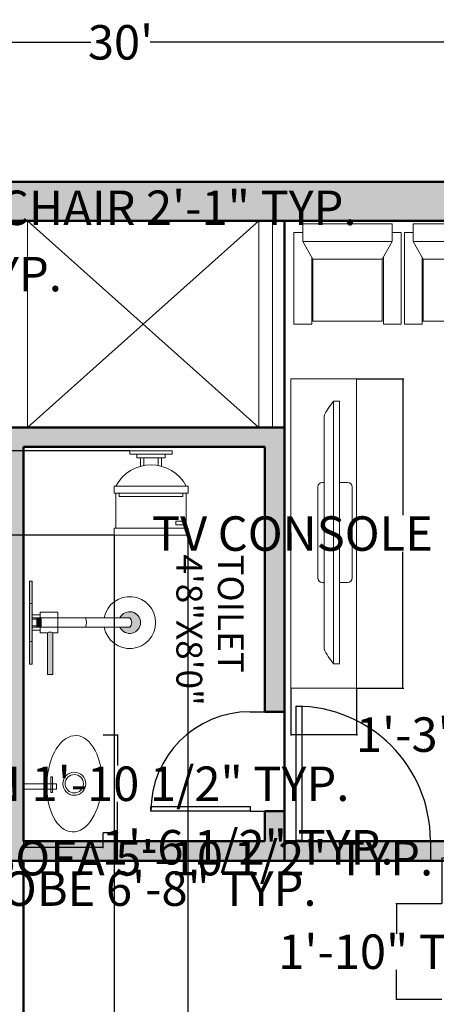
# Model space of a CAD drawing. Units: inches. Extents: x 22042254 to 25404563, y 17568978 to 17626777.
# Tile 43 of 45: x 22179940 to 22180037, y 17626547 to 17626775. Entities that reach past the tile are written whole.
import ezdxf

# ---------------------------------------------------------------- set-up
doc = ezdxf.new("R2010")
doc.units = ezdxf.units.IN
doc.header["$MEASUREMENT"] = 0
for name, color, linetype, lineweight in [('A-ANNO-DIMS', 2, 'Continuous', 18), ('A-AREA-IDEN', 7, 'Continuous', 18), ('A-FLOR-OPEN', 252, 'Continuous', 18), ('A-WALL-PATT', 244, 'Continuous', 13), ('doors', 4, 'Continuous', 25), ('furniture', 8, 'Continuous', 18), ('PLUMBING FIXTURES', 9, 'Continuous', 18), ('walls', 252, 'Continuous', 50)]:
    doc.layers.add(name, color=color, linetype=linetype, lineweight=lineweight)
doc.styles.get("Standard").update_dxf_attribs({"font": 'arial.ttf'})
doc.dimstyles.get("Standard").update_dxf_attribs({"dimtxt": 8, "dimasz": 0.18, "dimexe": 0.18, "dimexo": 0.0625, "dimgap": 0.09, "dimtad": 0, "dimtih": 1, "dimtoh": 1, "dimzin": 0, "dimdsep": 46, "dimlunit": 3, "dimtxsty": 'Standard', "dimcen": 0.09, "dimadec": 0, "dimazin": 0, "dimtfac": 1, "dimtofl": 0, "dimtmove": 0, "dimatfit": 3, "dimfxl": 1, "dimtolj": 1, "dimtzin": 0, "dimarcsym": 0})

# ---------------------------------------------------------------- blocks, each defined once
blk = doc.blocks.new('*D1')
at = {"layer": 'A-ANNO-DIMS', "color": 0, "lineweight": -2, "transparency": 16777216}
for p, q in [((22179783.73, 17626737.84), (22179783.73, 17626770.35)), ((22179783.91, 17626770.17), (22179956.86, 17626770.17)), ((22180143.55, 17626770.17), (22179970.61, 17626770.17)), ((22180143.73, 17626737.84), (22180143.73, 17626770.35))]:
    blk.add_line(p, q, dxfattribs=at)
at = {"layer": 'A-ANNO-DIMS', "color": 0, "transparency": 16777216}
for points in [[(22179783.91, 17626770.2), (22179783.91, 17626770.14), (22179783.73, 17626770.17)], [(22180143.55, 17626770.2), (22180143.55, 17626770.14), (22180143.73, 17626770.17)]]:
    blk.add_solid(points, dxfattribs=at)
at = {"layer": 'Defpoints', "color": 0, "transparency": 16777216}
for p in [(22180143.73, 17626770.17), (22179783.73, 17626737.78), (22180143.73, 17626737.78)]:
    blk.add_point(p, dxfattribs=at)
at = {"layer": 'A-ANNO-DIMS', "color": 0, "transparency": 16777216, "insert": (22179963.73, 17626770.17), "char_height": 8, "attachment_point": 5}
blk.add_mtext("\\A1;30'", dxfattribs=at)
blk = doc.blocks.new('FABRIC SOFA 1S')
at = {"layer": 'furniture'}
for p, q in [((3, 18.12), (34, 18.12)), ((3, 15.12), (3, 18.12)), ((34, 12.12), (34, 18.12)), ((0, -15.12), (0, 15.12)), ((6, 15.12), (0, 15.12)), ((6, -15.12), (6, 15.12)), ((12, 11.75), (6, 15.12)), ((11.33, 12.12), (34, 12.12)), ((6, -15.12), (12, -11.75)), ((11.33, -12.12), (34, -12.12)), ((34, -12.12), (34, -18.12)), ((6, -15.12), (0, -15.12)), ((3, -18.12), (3, -15.12)), ((3, -18.12), (34, -18.12))]:
    blk.add_line(p, q, dxfattribs=at)
blk.add_lwpolyline([(12, -11.75), (12, 11.75), (33, 11.75), (33, -11.75)], close=True, dxfattribs=at)
blk = doc.blocks.new('O.H SHOWER-PL')
at = {"layer": 'PLUMBING FIXTURES'}
for points in [[(-1.838, 0), (-1.838, -0.25), (1.838, -0.25), (1.838, 0)], [(0.461, -8.724), (0.461, -9.667, -0.422337), (-0.461, -9.667), (-0.461, -8.724, 4.325472)]]:
    blk.add_hatch(color=256, dxfattribs=at).paths.add_polyline_path(points)
for p, q in [((-1.838, 0), (-1.838, -0.25)), ((1.838, 0), (-1.838, 0)), ((1.838, 0), (1.838, -0.25)), ((1.838, -0.25), (-1.838, -0.25)), ((-0.461, -0.25), (-0.461, -9.667)), ((0.461, -0.25), (0.461, -9.667))]:
    blk.add_line(p, q, dxfattribs=at)
for centre, radius, start, end in [((0, -4.479), 1.033, 243.52996, 296.47004), ((0, -9.667), 2.501, 100.61004, 79.38997), ((0, -9.667), 1.049, 116.03487, 63.96515), ((0, -9.219), 0.643, 224.20776, 315.79224)]:
    blk.add_arc(centre, radius, start, end, dxfattribs=at)
blk = doc.blocks.new('DIVERTER-PL')
at = {"layer": 'PLUMBING FIXTURES'}
for points in [[(4, 0), (-4, 0), (-4, -0.25), (4, -0.25)], [(0.375, -1.144), (0.375, -0.704), (-0.375, -0.704), (-0.375, -1.144)], [(1, -1.751, 0.30818), (1, -2.251), (5, -2.251), (5, -1.751)]]:
    blk.add_hatch(color=256, dxfattribs=at).paths.add_polyline_path(points)
for p, q in [((-4, 0), (-4, -0.25)), ((-4, 0), (4, 0)), ((4, 0), (4, -0.25)), ((-4, -0.25), (4, -0.25)), ((-4, -0.25), (4, -0.25)), ((-0.75, -0.25), (-0.75, -1.05)), ((-0.375, -0.704), (0.375, -0.704)), ((-0.375, -0.704), (-0.375, -1.144)), ((-0.318, -0.704), (-0.318, -0.25)), ((0.318, -0.704), (0.318, -0.25)), ((0.375, -0.704), (0.375, -1.144)), ((0.75, -0.25), (0.75, -1.05)), ((-1, -1.05), (-0.375, -1.05)), ((-1, -1.05), (-1, -2.75)), ((-0.375, -1.144), (0.375, -1.144)), ((0.375, -1.05), (1, -1.05)), ((1, -1.05), (1, -1.751)), ((-1, -2.75), (1, -2.75)), ((1, -2.251), (1, -2.75))]:
    blk.add_line(p, q, dxfattribs=at)
at = {"layer": 'PLUMBING FIXTURES', "ltscale": 12}
for p, q in [((1, -1.751), (5, -1.751)), ((5, -2.251), (5, -1.751)), ((1, -2.251), (5, -2.251))]:
    blk.add_line(p, q, dxfattribs=at)
at = {"layer": 'PLUMBING FIXTURES'}
blk.add_arc((1.367, -2.001), 0.444, 145.74346, 214.25654, dxfattribs=at)
blk = doc.blocks.new('A$C7F153053')
at = {"layer": 'PLUMBING FIXTURES', "xscale": -1, "rotation": 270}
for name in ['DIVERTER-PL', 'O.H SHOWER-PL']:
    blk.add_blockref(name, (12.166, 4), dxfattribs=at)
blk = doc.blocks.new('Toilet - Imperial')
for p, q in [((-10, 22), (-10, 12)), ((-10, 21), (-7, 21)), ((-7, 20), (-10, 20)), ((-7, 21), (-7, 20)), ((10, 12), (10, 22)), ((10.5, 12), (-10.5, 12)), ((-10.5, 10), (-10.5, 12)), ((9, 13), (-9, 13)), ((-9, 13), (-9, 12)), ((9, 12), (9, 13)), ((10.5, 12), (10.5, 10)), ((10.5, 10), (-10.5, 10)), ((-3, 4.4065), (-3, 2)), ((-2, 2), (-2, 4.1658)), ((2, 4.1658), (2, 2)), ((3, 2), (3, 4.4065)), ((4, 2), (-4, 2)), ((-4, 2), (-4, 1)), ((4, 1), (4, 2))]:
    blk.add_line(p, q)
for points in [[(10.5, 22), (10.5, 24), (-10.5, 24), (-10.5, 22)], [(6, 0), (6, 1), (-6, 1), (-6, 0)]]:
    blk.add_lwpolyline(points, close=True)
blk.add_arc((0, 15.3333), 11.3333, 208.0725, 331.9275)
blk = doc.blocks.new('*U24')
for p, q in [((0, 0), (0, -6)), ((40, 0), (40, -6))]:
    blk.add_line(p, q)
blk.add_lwpolyline([(0, 0), (0, 40), (1.75, 40), (1.75, 0)], close=True)
blk.add_arc((0, 0), 40, 0, 90)
blk = doc.blocks.new('BASIN-OVAL-WITH-TAP')
for p, q in [((-11.77, 0), (-4.13, 0)), ((-5.47, 1.62), (-5.47, -2.04)), ((-5.06, 1.61), (-5.47, 1.61)), ((-5.06, -2.04), (-5.06, 1.61)), ((-4.13, 0), (-4.13, -1.24)), ((-4.13, -1.24), (-11.77, -1.24)), ((-5.47, -2.04), (-5.06, -2.04))]:
    blk.add_line(p, q)
for radius in [2.67, 2.13, 2.13, 2.13]:
    blk.add_circle((0, 0), radius)
blk.add_ellipse((0, 0), major_axis=(-0.46, -11.19), ratio=0.56899)
blk = doc.blocks.new('PLASMA-LARGE')
at = {"layer": 'furniture'}
for p, q in [((-7.26, 0), (7.26, 0)), ((-18.61, -1), (18.61, -1)), ((-8, -1), (-8, -0.74)), ((8, -1), (8, -0.74)), ((-21, -2.5), (21, -2.5)), ((-21, -2.5), (-21, -3.5)), ((21, -2.5), (21, -3.5)), ((-21, -3.5), (21, -3.5)), ((-8, -3.5), (-8, -4.76)), ((8, -3.5), (8, -4.76)), ((-7.26, -5.5), (7.26, -5.5))]:
    blk.add_line(p, q, dxfattribs=at)
for centre, radius, start, end in [((-7.26, -0.74), 0.744, 90, 180), ((7.26, -0.74), 0.744, 0, 90), ((-13.97, -11.05), 11.07, 114.7602, 129.4175), ((13.97, -11.05), 11.07, 50.5825, 65.2398), ((-7.26, -4.76), 0.744, 180, 270), ((7.26, -4.76), 0.744, 270, 0)]:
    blk.add_arc(centre, radius, start, end, dxfattribs=at)
blk = doc.blocks.new('TV-CONSOLE')
for p, q in [((8.99, 35.63), (-6.22, 35.63)), ((-6.22, 35.63), (-6.22, -36.14)), ((8.99, -36.14), (8.99, 35.63)), ((-6.22, -36.14), (8.99, -36.14))]:
    blk.add_line(p, q)
at = {"xscale": 1.450199298177205, "yscale": 1.450199298177205, "zscale": 1.450199298177205, "rotation": 90}
blk.add_blockref('PLASMA-LARGE', (0, 0), dxfattribs=at)
blk = doc.blocks.new('*D36')
at = {"layer": 'A-ANNO-DIMS', "color": 0, "lineweight": -2, "transparency": 16777216}
for p, q in [((22179884.69, 17626728.11), (22179884.69, 17626731.96)), ((22179884.87, 17626731.78), (22179909.36, 17626731.78)), ((22179909.54, 17626728.11), (22179909.54, 17626731.96)), ((22179909.54, 17626731.78), (22179909.72, 17626731.78))]:
    blk.add_line(p, q, dxfattribs=at)
at = {"layer": 'A-ANNO-DIMS', "color": 0, "transparency": 16777216}
for points in [[(22179884.87, 17626731.81), (22179884.87, 17626731.75), (22179884.69, 17626731.78)], [(22179909.36, 17626731.81), (22179909.36, 17626731.75), (22179909.54, 17626731.78)]]:
    blk.add_solid(points, dxfattribs=at)
at = {"layer": 'Defpoints', "color": 0, "transparency": 16777216}
for p in [(22179909.54, 17626731.78), (22179884.69, 17626728.05), (22179909.54, 17626728.05)]:
    blk.add_point(p, dxfattribs=at)
at = {"layer": 'A-ANNO-DIMS', "color": 0, "transparency": 16777216, "insert": (22179965.78, 17626731.78), "char_height": 8, "attachment_point": 5}
blk.add_mtext('\\A1;ARMCHAIR 2\'-1" TYP.', dxfattribs=at)
blk = doc.blocks.new('*D37')
at = {"layer": 'A-ANNO-DIMS', "color": 0, "lineweight": -2, "transparency": 16777216}
for p, q in [((22179909.6, 17626728.05), (22179913.44, 17626728.05)), ((22179913.26, 17626727.87), (22179913.26, 17626720.62)), ((22179913.26, 17626704.92), (22179913.26, 17626712.17)), ((22179909.6, 17626704.74), (22179913.44, 17626704.74))]:
    blk.add_line(p, q, dxfattribs=at)
at = {"layer": 'A-ANNO-DIMS', "color": 0, "transparency": 16777216}
for points in [[(22179913.23, 17626727.87), (22179913.29, 17626727.87), (22179913.26, 17626728.05)], [(22179913.23, 17626704.92), (22179913.29, 17626704.92), (22179913.26, 17626704.74)]]:
    blk.add_solid(points, dxfattribs=at)
at = {"layer": 'Defpoints', "color": 0, "transparency": 16777216}
for p in [(22179909.54, 17626728.05), (22179909.54, 17626704.74), (22179913.26, 17626704.74)]:
    blk.add_point(p, dxfattribs=at)
at = {"layer": 'A-ANNO-DIMS', "color": 0, "transparency": 16777216, "insert": (22179913.26, 17626716.39), "char_height": 8, "attachment_point": 5}
blk.add_mtext('\\A1;1\'-11 1/2" TYP.', dxfattribs=at)
blk = doc.blocks.new('*D38')
at = {"layer": 'A-ANNO-DIMS', "color": 0, "lineweight": -2, "transparency": 16777216}
for p, q in [((22180018.54, 17626692.07), (22180029.42, 17626692.07)), ((22180029.24, 17626691.89), (22180029.24, 17626660.42)), ((22180029.24, 17626620.49), (22180029.24, 17626651.96)), ((22180018.54, 17626620.31), (22180029.42, 17626620.31))]:
    blk.add_line(p, q, dxfattribs=at)
at = {"layer": 'A-ANNO-DIMS', "color": 0, "transparency": 16777216}
for points in [[(22180029.21, 17626691.89), (22180029.27, 17626691.89), (22180029.24, 17626692.07)], [(22180029.21, 17626620.49), (22180029.27, 17626620.49), (22180029.24, 17626620.31)]]:
    blk.add_solid(points, dxfattribs=at)
at = {"layer": 'Defpoints', "color": 0, "transparency": 16777216}
for p in [(22180018.48, 17626692.07), (22180029.24, 17626692.07), (22180018.48, 17626620.31)]:
    blk.add_point(p, dxfattribs=at)
at = {"layer": 'A-ANNO-DIMS', "color": 0, "transparency": 16777216, "insert": (22180029.24, 17626656.19), "char_height": 8, "attachment_point": 5}
blk.add_mtext('\\A1;TV CONSOLE 6\'-0" TYP.', dxfattribs=at)
blk = doc.blocks.new('*D39')
at = {"layer": 'A-ANNO-DIMS', "color": 0, "lineweight": -2, "transparency": 16777216}
for p, q in [((22180003.26, 17626620.25), (22180003.26, 17626609.36)), ((22180018.48, 17626620.25), (22180018.48, 17626609.36)), ((22180003.44, 17626609.54), (22180018.3, 17626609.54)), ((22180018.48, 17626609.54), (22180018.66, 17626609.54))]:
    blk.add_line(p, q, dxfattribs=at)
at = {"layer": 'A-ANNO-DIMS', "color": 0, "transparency": 16777216}
for points in [[(22180003.44, 17626609.57), (22180003.44, 17626609.51), (22180003.26, 17626609.54)], [(22180018.3, 17626609.57), (22180018.3, 17626609.51), (22180018.48, 17626609.54)]]:
    blk.add_solid(points, dxfattribs=at)
at = {"layer": 'Defpoints', "color": 0, "transparency": 16777216}
for p in [(22180003.26, 17626620.31), (22180018.48, 17626620.31), (22180018.48, 17626609.54)]:
    blk.add_point(p, dxfattribs=at)
at = {"layer": 'A-ANNO-DIMS', "color": 0, "transparency": 16777216, "insert": (22180042.75, 17626609.54), "char_height": 8, "attachment_point": 5}
blk.add_mtext('\\A1;1\'-3" TYP.', dxfattribs=at)
blk = doc.blocks.new('*D42')
at = {"layer": 'A-ANNO-DIMS', "color": 0, "lineweight": -2, "transparency": 16777216}
for p, q in [((22179814.6, 17626585.75), (22179814.6, 17626573.62)), ((22179894.63, 17626585.75), (22179894.63, 17626573.62)), ((22179814.78, 17626573.8), (22179894.45, 17626573.8)), ((22179894.63, 17626573.8), (22179894.81, 17626573.8))]:
    blk.add_line(p, q, dxfattribs=at)
at = {"layer": 'A-ANNO-DIMS', "color": 0, "transparency": 16777216}
for points in [[(22179814.78, 17626573.83), (22179814.78, 17626573.77), (22179814.6, 17626573.8)], [(22179894.45, 17626573.83), (22179894.45, 17626573.77), (22179894.63, 17626573.8)]]:
    blk.add_solid(points, dxfattribs=at)
at = {"layer": 'Defpoints', "color": 0, "transparency": 16777216}
for p in [(22179814.6, 17626585.81), (22179894.63, 17626585.81), (22179894.63, 17626573.8)]:
    blk.add_point(p, dxfattribs=at)
at = {"layer": 'A-ANNO-DIMS', "color": 0, "transparency": 16777216, "insert": (22179953.9, 17626573.8), "char_height": 8, "attachment_point": 5}
blk.add_mtext('\\A1;WARDROBE 6\'-8" TYP.', dxfattribs=at)
blk = doc.blocks.new('*D46')
at = {"layer": 'A-ANNO-DIMS', "color": 0, "lineweight": -2, "transparency": 16777216}
for p, q in [((22179959.69, 17626609.47), (22179963.21, 17626609.47)), ((22179963.03, 17626609.29), (22179963.03, 17626602.36)), ((22179963.03, 17626586.98), (22179963.03, 17626593.91)), ((22179959.69, 17626586.8), (22179963.21, 17626586.8))]:
    blk.add_line(p, q, dxfattribs=at)
at = {"layer": 'A-ANNO-DIMS', "color": 0, "transparency": 16777216}
for points in [[(22179963, 17626609.29), (22179963.06, 17626609.29), (22179963.03, 17626609.47)], [(22179963, 17626586.98), (22179963.06, 17626586.98), (22179963.03, 17626586.8)]]:
    blk.add_solid(points, dxfattribs=at)
at = {"layer": 'Defpoints', "color": 0, "transparency": 16777216}
for p in [(22179959.63, 17626609.47), (22179963.03, 17626609.47), (22179959.63, 17626586.8)]:
    blk.add_point(p, dxfattribs=at)
at = {"layer": 'A-ANNO-DIMS', "color": 0, "transparency": 16777216, "insert": (22179963.03, 17626598.14), "char_height": 8, "attachment_point": 5}
blk.add_mtext('\\A1;BASIN 1\'-10 1/2" TYP.', dxfattribs=at)
blk = doc.blocks.new('*D47')
at = {"layer": 'A-ANNO-DIMS', "color": 0, "lineweight": -2, "transparency": 16777216}
for p, q in [((22179941.23, 17626586.74), (22179941.23, 17626583.22)), ((22179959.63, 17626586.74), (22179959.63, 17626583.22)), ((22179941.41, 17626583.4), (22179959.45, 17626583.4)), ((22179959.63, 17626583.4), (22179959.81, 17626583.4))]:
    blk.add_line(p, q, dxfattribs=at)
at = {"layer": 'A-ANNO-DIMS', "color": 0, "transparency": 16777216}
for points in [[(22179941.41, 17626583.43), (22179941.41, 17626583.37), (22179941.23, 17626583.4)], [(22179959.45, 17626583.43), (22179959.45, 17626583.37), (22179959.63, 17626583.4)]]:
    blk.add_solid(points, dxfattribs=at)
at = {"layer": 'Defpoints', "color": 0, "transparency": 16777216}
for p in [(22179941.23, 17626586.8), (22179959.63, 17626586.8), (22179959.63, 17626583.4)]:
    blk.add_point(p, dxfattribs=at)
at = {"layer": 'A-ANNO-DIMS', "color": 0, "transparency": 16777216, "insert": (22179993.22, 17626583.4), "char_height": 8, "attachment_point": 5}
blk.add_mtext('\\A1;1\'-6 1/2" TYP.', dxfattribs=at)
blk = doc.blocks.new('*D48')
at = {"layer": 'A-ANNO-DIMS', "color": 0, "lineweight": -2, "transparency": 16777216}
for p, q in [((22180038.35, 17626580.87), (22180038.17, 17626580.87)), ((22180038.35, 17626570.34), (22180038.35, 17626581.05)), ((22180108.78, 17626580.87), (22180038.53, 17626580.87)), ((22180108.96, 17626570.34), (22180108.96, 17626581.05))]:
    blk.add_line(p, q, dxfattribs=at)
at = {"layer": 'A-ANNO-DIMS', "color": 0, "transparency": 16777216}
for points in [[(22180038.53, 17626580.9), (22180038.53, 17626580.84), (22180038.35, 17626580.87)], [(22180108.78, 17626580.9), (22180108.78, 17626580.84), (22180108.96, 17626580.87)]]:
    blk.add_solid(points, dxfattribs=at)
at = {"layer": 'Defpoints', "color": 0, "transparency": 16777216}
for p in [(22180038.35, 17626580.87), (22180038.35, 17626570.27), (22180108.96, 17626570.27)]:
    blk.add_point(p, dxfattribs=at)
at = {"layer": 'A-ANNO-DIMS', "color": 0, "transparency": 16777216, "insert": (22179984.52, 17626580.87), "char_height": 8, "attachment_point": 5}
blk.add_mtext('\\A1;SOFA 5\'-10 1/2" TYP.', dxfattribs=at)
blk = doc.blocks.new('*D49')
at = {"layer": 'A-ANNO-DIMS', "color": 0, "lineweight": -2, "transparency": 16777216}
for p, q in [((22180038.29, 17626570.27), (22180027.58, 17626570.27)), ((22180027.76, 17626570.09), (22180027.76, 17626563.33)), ((22180027.76, 17626548.22), (22180027.76, 17626554.98)), ((22180038.29, 17626548.04), (22180027.58, 17626548.04))]:
    blk.add_line(p, q, dxfattribs=at)
at = {"layer": 'A-ANNO-DIMS', "color": 0, "transparency": 16777216}
for points in [[(22180027.73, 17626570.09), (22180027.79, 17626570.09), (22180027.76, 17626570.27)], [(22180027.73, 17626548.22), (22180027.79, 17626548.22), (22180027.76, 17626548.04)]]:
    blk.add_solid(points, dxfattribs=at)
at = {"layer": 'Defpoints', "color": 0, "transparency": 16777216}
for p in [(22180038.35, 17626570.27), (22180027.76, 17626548.04), (22180038.35, 17626548.04)]:
    blk.add_point(p, dxfattribs=at)
at = {"layer": 'A-ANNO-DIMS', "color": 0, "transparency": 16777216, "insert": (22180027.76, 17626559.16), "char_height": 8, "attachment_point": 5}
blk.add_mtext('\\A1;1\'-10" TYP.', dxfattribs=at)
blk = doc.blocks.new('*D62')
at = {"layer": 'A-ANNO-DIMS', "color": 0, "lineweight": -2, "transparency": 16777216}
for p, q in [((22179965.84, 17626675.39), (22179727.35, 17626675.39)), ((22179727.53, 17626675.21), (22179727.53, 17626669.81)), ((22179727.53, 17626655.96), (22179727.53, 17626661.36)), ((22179962.16, 17626655.78), (22179727.35, 17626655.78))]:
    blk.add_line(p, q, dxfattribs=at)
at = {"layer": 'A-ANNO-DIMS', "color": 0, "transparency": 16777216}
for points in [[(22179727.5, 17626675.21), (22179727.56, 17626675.21), (22179727.53, 17626675.39)], [(22179727.5, 17626655.96), (22179727.56, 17626655.96), (22179727.53, 17626655.78)]]:
    blk.add_solid(points, dxfattribs=at)
at = {"layer": 'Defpoints', "color": 0, "transparency": 16777216}
for p in [(22179965.9, 17626675.39), (22179727.53, 17626655.78), (22179962.22, 17626655.78)]:
    blk.add_point(p, dxfattribs=at)
at = {"layer": 'A-ANNO-DIMS', "color": 0, "transparency": 16777216, "insert": (22179727.53, 17626665.59), "char_height": 8, "attachment_point": 5}
blk.add_mtext('\\A1;1\'-7 1/2"', dxfattribs=at)
blk = doc.blocks.new('*D63')
at = {"layer": 'A-ANNO-DIMS', "color": 0, "lineweight": -2, "transparency": 16777216}
for p, q in [((22179962.22, 17626655.72), (22179962.22, 17626158.2)), ((22179979.38, 17626655.72), (22179979.38, 17626158.2)), ((22179962.4, 17626158.38), (22179979.2, 17626158.38)), ((22179979.38, 17626158.38), (22179979.56, 17626158.38))]:
    blk.add_line(p, q, dxfattribs=at)
at = {"layer": 'A-ANNO-DIMS', "color": 0, "transparency": 16777216}
for points in [[(22179962.4, 17626158.41), (22179962.4, 17626158.35), (22179962.22, 17626158.38)], [(22179979.2, 17626158.41), (22179979.2, 17626158.35), (22179979.38, 17626158.38)]]:
    blk.add_solid(points, dxfattribs=at)
at = {"layer": 'Defpoints', "color": 0, "transparency": 16777216}
for p in [(22179962.22, 17626655.78), (22179979.38, 17626655.78), (22179979.38, 17626158.38)]:
    blk.add_point(p, dxfattribs=at)
at = {"layer": 'A-ANNO-DIMS', "color": 0, "transparency": 16777216, "insert": (22179989.91, 17626158.38), "char_height": 8, "attachment_point": 5}
blk.add_mtext('\\A1;1\'-5"', dxfattribs=at)

msp = doc.modelspace()

# ---------------------------------------------------------------- hatches: boundary and pattern name
at = {"layer": 'A-WALL-PATT'}
h = msp.add_hatch(color=256, dxfattribs=at)
h.dxf.hatch_style = 1
h.paths.add_polyline_path([(22179792.734, 17626580.28), (22179888.734, 17626580.28), (22179888.734, 17626559.623), (22179893.234, 17626559.623), (22179893.234, 17626580.28), (22179900.438, 17626580.28), (22179900.438, 17626584.78), (22179792.734, 17626584.78), (22179792.734, 17626728.78), (22180134.734, 17626728.78), (22180134.734, 17626584.78), (22180035.602, 17626584.78), (22180004.432, 17626584.78), (22180001.734, 17626584.78), (22180001.734, 17626580.28), (22180134.734, 17626580.28), (22180134.734, 17626404.28), (22180064.487, 17626404.28), (22180064.487, 17626399.78), (22180134.734, 17626399.78), (22180134.734, 17626197.78), (22180143.734, 17626197.78), (22180143.734, 17626737.78), (22179783.734, 17626737.78), (22179783.734, 17626197.78), (22179792.734, 17626197.78), (22179792.734, 17626394.78), (22179936.734, 17626394.78), (22179936.734, 17626383.208), (22179941.234, 17626383.208), (22179941.234, 17626532.28), (22179927.066, 17626532.28), (22179927.066, 17626527.78), (22179928.072, 17626527.78), (22179936.734, 17626527.78), (22179936.734, 17626403.78), (22179792.734, 17626403.78), (22179792.734, 17626527.78), (22179905.094, 17626527.78), (22179905.094, 17626532.28), (22179792.734, 17626532.28)])
h = msp.add_hatch(color=256, dxfattribs=at)
h.dxf.hatch_style = 1
h.paths.add_polyline_path([(22179941.234, 17626676.28), (22179997.234, 17626676.28), (22179997.234, 17626614.838), (22180001.734, 17626614.838), (22180001.734, 17626680.78), (22179936.734, 17626680.78), (22179936.734, 17626617.551), (22179936.734, 17626580.28), (22179941.234, 17626580.28), (22180001.734, 17626580.28), (22180001.734, 17626591.815), (22179997.234, 17626591.815), (22179997.234, 17626584.78), (22179941.234, 17626584.78)])
h = msp.add_hatch(color=256, dxfattribs=at)
h.dxf.hatch_style = 1
h.paths.add_polyline_path([(22180004.432, 17626584.78), (22180001.734, 17626584.78), (22180001.734, 17626580.28), (22180004.432, 17626580.28)])
h.paths.add_polyline_path([(22179975.057, 17626652.876), (22179975.057, 17626616.493), (22179984.229, 17626616.493), (22179984.229, 17626652.876)], flags=9)
h.paths.add_polyline_path([(22179984.656, 17626652.896), (22179984.656, 17626620.513), (22179993.952, 17626620.513), (22179993.952, 17626652.896)], flags=9)

# ---------------------------------------------------------------- linework, layer by layer
at = {"layer": 'A-FLOR-OPEN'}
for p, q in [((22179942.159, 17626728.78), (22179942.159, 17626680.78)), ((22179942.159, 17626728.78), (22179995.774, 17626680.78)), ((22179942.159, 17626680.78), (22179995.774, 17626728.78)), ((22179995.774, 17626728.78), (22179995.774, 17626680.78)), ((22179998.968, 17626680.78), (22179998.968, 17626728.78))]:
    msp.add_line(p, q, dxfattribs=at)
at = {"layer": 'walls'}
for p, q in [((22179783.734, 17626737.78), (22180143.734, 17626737.78)), ((22179792.734, 17626728.78), (22180134.734, 17626728.78)), ((22180001.734, 17626580.28), (22180001.734, 17626728.78)), ((22179936.734, 17626680.78), (22180001.734, 17626680.78)), ((22179941.234, 17626676.28), (22179997.234, 17626676.28)), ((22179941.234, 17626584.78), (22179941.234, 17626676.28)), ((22179997.234, 17626614.838), (22179997.234, 17626676.28)), ((22179997.234, 17626614.838), (22180001.734, 17626614.838)), ((22179997.234, 17626584.78), (22179997.234, 17626591.815)), ((22179997.234, 17626591.815), (22180001.734, 17626591.815)), ((22179941.234, 17626584.78), (22179997.234, 17626584.78)), ((22180001.734, 17626584.78), (22180004.432, 17626584.78)), ((22180004.432, 17626584.78), (22180035.602, 17626584.78)), ((22180035.602, 17626584.78), (22180134.734, 17626584.78)), ((22179893.234, 17626580.28), (22179941.234, 17626580.28)), ((22179893.234, 17626580.28), (22180134.734, 17626580.28)), ((22179941.234, 17626532.28), (22179941.234, 17626580.28))]:
    msp.add_line(p, q, dxfattribs=at)

# ---------------------------------------------------------------- block references
at = {"layer": 'doors', "xscale": 0.5755769432943251, "yscale": 0.5755769432943251, "zscale": 0.5755769432943251, "rotation": 90}
msp.add_blockref('*U24', (22179993.78, 17626591.815), dxfattribs=at)
at = {"layer": 'doors', "xscale": 0.7792671805443983, "yscale": 0.7792671805443983, "zscale": 0.7792671805443983}
msp.add_blockref('*U24', (22180004.432, 17626584.955), dxfattribs=at)
at = {"layer": 'furniture', "xscale": 0.685544738852578, "yscale": 0.685544738852578, "zscale": 0.685544738852578, "rotation": 270}
for p in [(22180016.389, 17626728.088), (22180041.998, 17626728.088)]:
    msp.add_blockref('FABRIC SOFA 1S', p, dxfattribs=at)
at = {"layer": 'furniture'}
msp.add_blockref('TV-CONSOLE', (22180009.482, 17626656.443), dxfattribs=at)
at = {"layer": 'PLUMBING FIXTURES', "rotation": 180}
for name, p, xscale, yscale, zscale in [('Toilet - Imperial', (22179970.804, 17626675.394), 0.8171681656610218, 0.8171681656610218, 0.8171681656610218), ('A$C7F153053', (22179971.872, 17626645.17), 2.406230429091579, 2.406230429091579, 2.406230429091579)]:
    msp.add_blockref(name, p, dxfattribs=dict(at, xscale=xscale, yscale=yscale, zscale=zscale))
at = {"layer": 'PLUMBING FIXTURES'}
msp.add_blockref('BASIN-OVAL-WITH-TAP', (22179953.006, 17626598.136), dxfattribs=at)

# ---------------------------------------------------------------- texts
at = {"layer": 'A-AREA-IDEN'}
for s, p in [('4\'8"X8\'0"', (22179976.688, 17626651.347)), ('TOILET', (22179986.308, 17626651.347))]:
    msp.add_text(s, height=5.9886, rotation=270, dxfattribs=at).set_placement(p)

# ---------------------------------------------------------------- dimensions: what is measured, and where the dimension line sits
at = {"layer": 'A-ANNO-DIMS'}
for base, p1, p2, override, picture, middle in [((22180143.734, 17626770.174), (22179783.734, 17626737.78), (22180143.734, 17626737.78), {"dimclrd": 0, "dimclre": 0, "dimclrt": 0}, '*D1', (22179963.734, 17626770.174)), ((22179979.384, 17626158.384), (22179962.224, 17626655.782), (22179979.384, 17626655.782), {"dimdec": 1, "dimlfac": 1, "dimrnd": 0, "dimzin": 1, "dimdsep": 46, "dimlunit": 4, "dimfrac": 2}, '*D63', (22179989.911, 17626158.384))]:
    dim = msp.add_linear_dim(base=base, p1=p1, p2=p2, dimstyle='Standard', override=override, dxfattribs=at)
    dim.commit()
    dim.dimension.update_dxf_attribs({"geometry": picture, "text_midpoint": middle})
for base, p1, p2, text, picture, middle in [((22179909.537, 17626731.776), (22179884.686, 17626728.048), (22179909.537, 17626728.048), 'ARMCHAIR <> TYP.', '*D36', (22179965.777, 17626731.776)), ((22180018.476, 17626609.543), (22180003.262, 17626620.308), (22180018.476, 17626620.308), '<> TYP.', '*D39', (22180042.751, 17626609.543)), ((22179959.629, 17626583.397), (22179941.234, 17626586.798), (22179959.629, 17626586.798), '<> TYP.', '*D47', (22179993.225, 17626583.397)), ((22179894.625, 17626573.805), (22179814.602, 17626585.808), (22179894.625, 17626585.808), 'WARDROBE <> TYP.', '*D42', (22179953.902, 17626573.805))]:
    dim = msp.add_linear_dim(base=base, p1=p1, p2=p2, text=text, dimstyle='Standard', override={"dimdec": 1, "dimlfac": 1, "dimrnd": 0, "dimzin": 1, "dimdsep": 46, "dimlunit": 4, "dimfrac": 2}, dxfattribs=at)
    dim.commit()
    dim.dimension.update_dxf_attribs({"geometry": picture, "text_midpoint": middle})
for base, p1, p2, angle, text, picture, middle in [((22179913.265, 17626704.74), (22179909.537, 17626728.048), (22179909.537, 17626704.74), 270, '<> TYP.', '*D37', (22179913.265, 17626716.394)), ((22180029.241, 17626692.074), (22180018.476, 17626620.308), (22180018.476, 17626692.074), 90, 'TV CONSOLE <> TYP.', '*D38', (22180029.241, 17626656.191)), ((22179963.03, 17626609.475), (22179959.629, 17626586.798), (22179959.629, 17626609.475), 90, 'BASIN <> TYP.', '*D46', (22179963.03, 17626598.136)), ((22180038.35, 17626580.865), (22180108.959, 17626570.274), (22180038.35, 17626570.274), 180, 'SOFA <> TYP.', '*D48', (22179984.522, 17626580.865)), ((22180027.758, 17626548.045), (22180038.35, 17626570.274), (22180038.35, 17626548.045), 270, '<> TYP.', '*D49', (22180027.758, 17626559.159))]:
    dim = msp.add_linear_dim(base=base, p1=p1, p2=p2, angle=angle, text=text, dimstyle='Standard', override={"dimdec": 1, "dimlfac": 1, "dimrnd": 0, "dimzin": 1, "dimdsep": 46, "dimlunit": 4, "dimfrac": 2}, dxfattribs=at)
    dim.commit()
    dim.dimension.update_dxf_attribs({"geometry": picture, "text_midpoint": middle})
dim = msp.add_linear_dim(base=(22179727.534, 17626655.782), p1=(22179965.901, 17626675.394), p2=(22179962.224, 17626655.782), angle=90, dimstyle='Standard', override={"dimdec": 1, "dimlfac": 1, "dimrnd": 0, "dimzin": 1, "dimdsep": 46, "dimlunit": 4, "dimfrac": 2}, dxfattribs=at)
dim.commit()
dim.dimension.update_dxf_attribs({"geometry": '*D62', "text_midpoint": (22179727.534, 17626665.588)})

doc.saveas('drawing.dxf')
